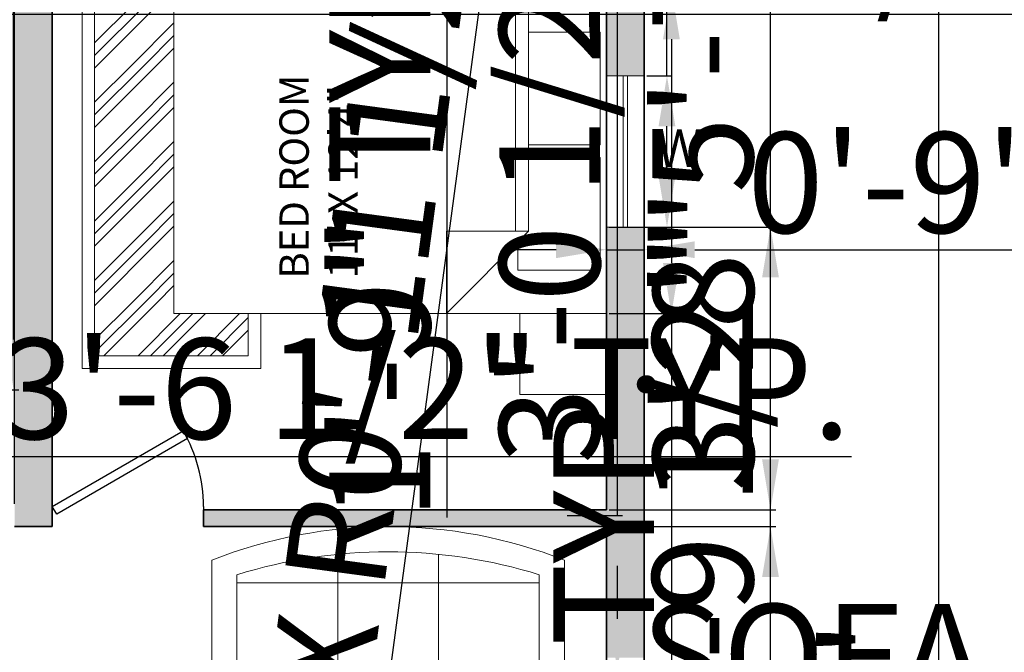
# Model space of a CAD drawing. Units: inches. Extents: x 830 to 1639, y 2591 to 3595.
# Tile 4 of 7: x 1133 to 1367, y 2957 to 3108. Entities that reach past the tile are written whole.
import ezdxf

# ---------------------------------------------------------------- set-up
doc = ezdxf.new("R2010")
doc.units = ezdxf.units.IN
doc.layers.get('0').update_dxf_attribs({"color": 250})
for name, color, linetype, lineweight in [('A-ANNO-DIMS', 2, 'Continuous', 18), ('A-ANNO-TEXT', 7, 'Continuous', 18), ('A-AREA-IDEN', 7, 'Continuous', 25), ('A-DOOR', 3, 'Continuous', 25), ('A-FLOR-PATT', 252, 'Continuous', 13), ('A-FURN', 8, 'Continuous', 18), ('A-GLAZ', 4, 'Continuous', 18), ('A-WALL', 7, 'Continuous', 35), ('A-WALL-PATT', 5, 'Continuous', 13), ('C-PROP', 7, 'Continuous', 35)]:
    doc.layers.add(name, color=color, linetype=linetype, lineweight=lineweight)
doc.styles.get("Standard").update_dxf_attribs({"font": 'arial.ttf'})
doc.dimstyles.new('ISO-25', dxfattribs={"dimtxt": 24, "dimasz": 12, "dimexe": 1.25, "dimexo": 0.625, "dimtad": 1, "dimdec": 0, "dimlunit": 3, "dimtxsty": 'Standard', "dimcen": 2.5, "dimadec": 0, "dimazin": 0, "dimtfac": 1, "dimtdec": 0, "dimtmove": 0, "dimatfit": 3, "dimfxl": 1, "dimarcsym": 0})

# ---------------------------------------------------------------- blocks, each defined once
blk = doc.blocks.new('Sofa - Roundback 7 ft.')
for p, q in [((-12.00002, -32.4421), (-12.00003, -6.5971)), ((11.99997, -32.4421), (11.99998, -6.5971)), ((-36.000027, -34), (-36.000027, -11.4696)), ((35.99998, -34), (35.99998, -11.4696)), ((-35.999844, -13.3819), (35.9998, -13.3819)), ((-36.000027, -32.4421), (35.99998, -32.4421))]:
    blk.add_line(p, q)
for points in [[(-36.000027, -34), (-42.000027, -34), (-42.000027, -8)], [(41.99998, -8), (41.99998, -34), (35.99998, -34)]]:
    blk.add_lwpolyline(points)
for centre, radius, start, end in [((0, -114.25), 114.25, 68.43141, 111.5686), ((-0.00001, -127.1968), 121.1968, 72.72033, 107.2797)]:
    blk.add_arc(centre, radius, start, end)
blk = doc.blocks.new('*U11')
for p, q in [((-750, 0), (-750, 100)), ((0, 0), (0, 100))]:
    blk.add_line(p, q)
blk.add_lwpolyline([(0, 0), (-649.5, -375), (-671.4, -337.1), (-21.9, 37.9)], close=True)
blk.add_arc((0, 0), 750, 180, 210)
blk = doc.blocks.new('Bed - Queen')
for p, q in [((0, -80.00003), (0, 0)), ((0, 0), (59.99999, 0)), ((59.99999, 0), (59.99999, -80.00003)), ((7.99999, -1.2), (28.79998, -1.2)), ((7.99999, -14.4), (7.99999, -1.2)), ((28.79998, -1.2), (28.79998, -14.4)), ((31.19999, -1.2), (51.99999, -1.2)), ((31.19999, -14.4), (31.19999, -1.2)), ((51.99999, -1.2), (51.99999, -16.4)), ((0, -14.4), (44.8, -14.4)), ((59.99999, -29.6), (44.8, -14.4)), ((44.8, -14.4), (44.8, -29.6)), ((44.8, -16.8), (0, -16.8)), ((51.99999, -16.4), (46.79936, -16.4)), ((44.8, -29.6), (59.99999, -29.6)), ((59.99999, -80.00003), (0, -80.00003))]:
    blk.add_line(p, q)
blk = doc.blocks.new('*D14')
at = {"layer": 'A-ANNO-DIMS', "color": 0, "lineweight": -2, "transparency": 16777216}
for p, q in [((1282.21, 3212.09), (1352.88, 3212.09)), ((1351.63, 3200.09), (1351.63, 2684.09)), ((1282.21, 2672.09), (1352.88, 2672.09))]:
    blk.add_line(p, q, dxfattribs=at)
at = {"layer": 'A-ANNO-DIMS', "color": 0, "transparency": 16777216}
for points in [[(1349.63, 3200.09), (1353.63, 3200.09), (1351.63, 3212.09)], [(1349.63, 2684.09), (1353.63, 2684.09), (1351.63, 2672.09)]]:
    blk.add_solid(points, dxfattribs=at)
at = {"layer": 'Defpoints', "color": 0, "transparency": 16777216}
for p in [(1281.59, 3212.09), (1281.59, 2672.09), (1351.63, 2672.09)]:
    blk.add_point(p, dxfattribs=at)
at = {"layer": 'A-ANNO-DIMS', "color": 0, "transparency": 16777216, "insert": (1338.8, 2942.09), "char_height": 24, "attachment_point": 5, "rotation": 90}
blk.add_mtext("45'", dxfattribs=at)
blk = doc.blocks.new('WIN-36IN')
for p, q in [((0, 0), (0, 36)), ((0, 36), (9, 36)), ((4, 0), (4, 36)), ((5, 36), (5, 0)), ((9, 36), (9, 0)), ((9, 0), (0, 0))]:
    blk.add_line(p, q)
blk = doc.blocks.new('BEDSIDE-TABLE')
blk.add_lwpolyline([(20.72, 0), (0, 0), (0, 19.25), (20.72, 19.25)], close=True)
blk = doc.blocks.new('BED-RUG-PLAN')
for points in [[(0, 92.63), (0, 105.69), (42.59, 105.69), (42.59, 0), (0, 0), (0, 15.31)], [(3, 92.63), (3, 102.69), (39.59, 102.69), (39.59, 3), (3, 3), (3, 15.31)]]:
    blk.add_lwpolyline(points)
blk = doc.blocks.new('*D22')
at = {"layer": 'A-ANNO-DIMS', "color": 0, "lineweight": -2, "transparency": 16777216}
for p, q in [((1286.99, 3094.42), (1286.99, 3411.37)), ((1282.21, 3094.42), (1288.24, 3094.42)), ((1286.99, 3070.42), (1286.99, 3082.42)), ((1282.21, 3058.42), (1288.24, 3058.42))]:
    blk.add_line(p, q, dxfattribs=at)
at = {"layer": 'A-ANNO-DIMS', "color": 0, "transparency": 16777216}
for points in [[(1284.99, 3082.42), (1288.99, 3082.42), (1286.99, 3094.42)], [(1284.99, 3070.42), (1288.99, 3070.42), (1286.99, 3058.42)]]:
    blk.add_solid(points, dxfattribs=at)
at = {"layer": 'Defpoints', "color": 0, "transparency": 16777216}
for p in [(1281.59, 3094.42), (1286.99, 3094.42), (1281.59, 3058.42)]:
    blk.add_point(p, dxfattribs=at)
at = {"layer": 'A-ANNO-DIMS', "color": 0, "transparency": 16777216, "insert": (1273.94, 3258.89), "char_height": 24, "attachment_point": 5, "rotation": 90}
blk.add_mtext('WINDOW 3\'-0" TYP.', dxfattribs=at)
blk = doc.blocks.new('*D23')
at = {"layer": 'A-ANNO-DIMS', "color": 0, "lineweight": -2, "transparency": 16777216}
for p, q in [((1272.59, 3057.79), (1272.59, 3051.77)), ((1281.59, 3057.79), (1281.59, 3051.77)), ((1260.59, 3053.02), (1248.59, 3053.02)), ((1272.59, 3053.02), (1281.59, 3053.02)), ((1293.59, 3053.02), (1453.13, 3053.02))]:
    blk.add_line(p, q, dxfattribs=at)
at = {"layer": 'A-ANNO-DIMS', "color": 0, "transparency": 16777216}
for points in [[(1260.59, 3055.02), (1260.59, 3051.02), (1272.59, 3053.02)], [(1293.59, 3055.02), (1293.59, 3051.02), (1281.59, 3053.02)]]:
    blk.add_solid(points, dxfattribs=at)
at = {"layer": 'Defpoints', "color": 0, "transparency": 16777216}
for p in [(1272.59, 3058.42), (1281.59, 3058.42), (1281.59, 3053.02)]:
    blk.add_point(p, dxfattribs=at)
at = {"layer": 'A-ANNO-DIMS', "color": 0, "transparency": 16777216, "insert": (1379.36, 3065.9), "char_height": 24, "attachment_point": 5}
blk.add_mtext('0\'-9" TYP.', dxfattribs=at)
blk = doc.blocks.new('*D26')
at = {"layer": 'A-ANNO-DIMS', "color": 0, "lineweight": -2, "transparency": 16777216}
for p, q in [((990.59, 3111.63), (990.59, 3107.9)), ((1011.31, 3111.63), (1011.31, 3107.9)), ((978.59, 3109.15), (966.59, 3109.15)), ((990.59, 3109.15), (1011.31, 3109.15)), ((1023.31, 3109.15), (1464.86, 3109.15))]:
    blk.add_line(p, q, dxfattribs=at)
at = {"layer": 'A-ANNO-DIMS', "color": 0, "transparency": 16777216}
for points in [[(978.59, 3111.15), (978.59, 3107.15), (990.59, 3109.15)], [(1023.31, 3111.15), (1023.31, 3107.15), (1011.31, 3109.15)]]:
    blk.add_solid(points, dxfattribs=at)
at = {"layer": 'Defpoints', "color": 0, "transparency": 16777216}
for p in [(990.59, 3112.26), (1011.31, 3112.26), (1011.31, 3109.15)]:
    blk.add_point(p, dxfattribs=at)
at = {"layer": 'A-ANNO-DIMS', "color": 0, "transparency": 16777216, "insert": (1250.08, 3122.18), "char_height": 24, "attachment_point": 5}
blk.add_mtext('NIGHTSTAND 1\'-8 1/2" TYP.', dxfattribs=at)
blk = doc.blocks.new('*D28')
at = {"layer": 'A-ANNO-DIMS', "color": 0, "lineweight": -2, "transparency": 16777216}
for p, q in [((1178.57, 2952.46), (1178.57, 2939.24)), ((1262.57, 2952.46), (1262.57, 2939.24)), ((1190.57, 2940.49), (1250.57, 2940.49)), ((1262.57, 2940.49), (1522.6, 2940.49))]:
    blk.add_line(p, q, dxfattribs=at)
at = {"layer": 'A-ANNO-DIMS', "color": 0, "transparency": 16777216}
for points in [[(1190.57, 2942.49), (1190.57, 2938.49), (1178.57, 2940.49)], [(1250.57, 2942.49), (1250.57, 2938.49), (1262.57, 2940.49)]]:
    blk.add_solid(points, dxfattribs=at)
at = {"layer": 'Defpoints', "color": 0, "transparency": 16777216}
for p in [(1178.57, 2953.09), (1262.57, 2953.09), (1262.57, 2940.49)]:
    blk.add_point(p, dxfattribs=at)
at = {"layer": 'A-ANNO-DIMS', "color": 0, "transparency": 16777216, "insert": (1398.58, 2953.53), "char_height": 24, "attachment_point": 5}
blk.add_mtext('SOFA 7\'-0" TYP.', dxfattribs=at)
blk = doc.blocks.new('*D29')
at = {"layer": 'A-ANNO-DIMS', "color": 0, "lineweight": -2, "transparency": 16777216}
for p, q in [((1275.17, 2989.75), (1275.17, 3205.2)), ((1263.19, 2989.75), (1276.42, 2989.75)), ((1275.17, 2965.09), (1275.17, 2977.75)), ((1263.19, 2953.09), (1276.42, 2953.09))]:
    blk.add_line(p, q, dxfattribs=at)
at = {"layer": 'A-ANNO-DIMS', "color": 0, "transparency": 16777216}
for points in [[(1273.17, 2977.75), (1277.17, 2977.75), (1275.17, 2989.75)], [(1273.17, 2965.09), (1277.17, 2965.09), (1275.17, 2953.09)]]:
    blk.add_solid(points, dxfattribs=at)
at = {"layer": 'Defpoints', "color": 0, "transparency": 16777216}
for p in [(1262.57, 2989.75), (1275.17, 2989.75), (1262.57, 2953.09)]:
    blk.add_point(p, dxfattribs=at)
at = {"layer": 'A-ANNO-DIMS', "color": 0, "transparency": 16777216, "insert": (1262.13, 3103.48), "char_height": 24, "attachment_point": 5, "rotation": 90}
blk.add_mtext('3\'-0 1/2" TYP.', dxfattribs=at)
blk = doc.blocks.new('*D31')
at = {"layer": 'A-ANNO-DIMS', "color": 0, "lineweight": -2, "transparency": 16777216}
for p, q in [((1234.59, 3191.58), (1234.59, 3203.58)), ((1238.92, 3179.58), (1233.34, 3179.58)), ((1234.59, 3179.58), (1234.59, 3158.58)), ((1238.92, 3158.58), (1233.34, 3158.58)), ((1234.59, 3146.58), (1234.59, 2989.29))]:
    blk.add_line(p, q, dxfattribs=at)
at = {"layer": 'A-ANNO-DIMS', "color": 0, "transparency": 16777216}
for points in [[(1232.59, 3191.58), (1236.59, 3191.58), (1234.59, 3179.58)], [(1232.59, 3146.58), (1236.59, 3146.58), (1234.59, 3158.58)]]:
    blk.add_solid(points, dxfattribs=at)
at = {"layer": 'Defpoints', "color": 0, "transparency": 16777216}
for p in [(1239.54, 3179.58), (1234.59, 3158.58), (1239.54, 3158.58)]:
    blk.add_point(p, dxfattribs=at)
at = {"layer": 'A-ANNO-DIMS', "color": 0, "transparency": 16777216, "insert": (1221.71, 3061.94), "char_height": 24, "attachment_point": 5, "rotation": 90}
blk.add_mtext('1\'-9" TYP.', dxfattribs=at)
blk = doc.blocks.new('*D36')
at = {"layer": 'A-ANNO-DIMS', "color": 0, "lineweight": -2, "transparency": 16777216}
for p, q in [((1169.49, 3115.77), (1169.49, 3131.86)), ((1272.59, 3115.77), (1272.59, 3131.86)), ((1181.49, 3130.61), (1260.59, 3130.61)), ((1272.59, 3130.61), (1638.88, 3130.61))]:
    blk.add_line(p, q, dxfattribs=at)
at = {"layer": 'A-ANNO-DIMS', "color": 0, "transparency": 16777216}
for points in [[(1181.49, 3132.61), (1181.49, 3128.61), (1169.49, 3130.61)], [(1260.59, 3132.61), (1260.59, 3128.61), (1272.59, 3130.61)]]:
    blk.add_solid(points, dxfattribs=at)
at = {"layer": 'Defpoints', "color": 0, "transparency": 16777216}
for p in [(1272.59, 3130.61), (1169.49, 3115.15), (1272.59, 3115.15)]:
    blk.add_point(p, dxfattribs=at)
at = {"layer": 'A-ANNO-DIMS', "color": 0, "transparency": 16777216, "insert": (1461.74, 3144.38), "char_height": 24, "attachment_point": 5}
blk.add_mtext('QUEEN BED 8\'-7" TYP.', dxfattribs=at)
blk = doc.blocks.new('*D37')
at = {"layer": 'A-ANNO-DIMS', "color": 0, "lineweight": -2, "transparency": 16777216}
for p, q in [((1273.21, 3115.15), (1289.3, 3115.15)), ((1288.05, 3103.15), (1288.05, 3049.83)), ((1273.21, 3037.83), (1289.3, 3037.83)), ((1288.05, 3037.83), (1288.05, 2822.23))]:
    blk.add_line(p, q, dxfattribs=at)
at = {"layer": 'A-ANNO-DIMS', "color": 0, "transparency": 16777216}
for points in [[(1286.05, 3103.15), (1290.05, 3103.15), (1288.05, 3115.15)], [(1286.05, 3049.83), (1290.05, 3049.83), (1288.05, 3037.83)]]:
    blk.add_solid(points, dxfattribs=at)
at = {"layer": 'Defpoints', "color": 0, "transparency": 16777216}
for p in [(1272.59, 3115.15), (1272.59, 3037.83), (1288.05, 3037.83)]:
    blk.add_point(p, dxfattribs=at)
at = {"layer": 'A-ANNO-DIMS', "color": 0, "transparency": 16777216, "insert": (1275.02, 2924.03), "char_height": 24, "attachment_point": 5, "rotation": 90}
blk.add_mtext('6\'-5 1/2" TYP.', dxfattribs=at)
blk = doc.blocks.new('*D39')
at = {"layer": 'A-ANNO-DIMS', "color": 0, "lineweight": -2, "transparency": 16777216}
for p, q in [((1209.62, 3142.46), (1209.62, 3139.14)), ((1220.27, 3142.46), (1220.27, 3139.14)), ((1197.62, 3140.39), (1185.62, 3140.39)), ((1209.62, 3140.39), (1220.27, 3140.39)), ((1232.27, 3140.39), (1466.38, 3140.39))]:
    blk.add_line(p, q, dxfattribs=at)
at = {"layer": 'A-ANNO-DIMS', "color": 0, "transparency": 16777216}
for points in [[(1197.62, 3142.39), (1197.62, 3138.39), (1209.62, 3140.39)], [(1232.27, 3142.39), (1232.27, 3138.39), (1220.27, 3140.39)]]:
    blk.add_solid(points, dxfattribs=at)
at = {"layer": 'Defpoints', "color": 0, "transparency": 16777216}
for p in [(1209.62, 3143.09), (1220.27, 3143.09), (1220.27, 3140.39)]:
    blk.add_point(p, dxfattribs=at)
at = {"layer": 'A-ANNO-DIMS', "color": 0, "transparency": 16777216, "insert": (1355.32, 3153.43), "char_height": 24, "attachment_point": 5}
blk.add_mtext('0\'-10 1/2" TYP.', dxfattribs=at)
blk = doc.blocks.new('*D40')
at = {"layer": 'A-ANNO-DIMS', "color": 0, "lineweight": -2, "transparency": 16777216}
for p, q in [((1131.38, 3125.32), (1131.38, 3423.36)), ((1116.15, 3125.32), (1132.63, 3125.32)), ((1131.38, 3031.63), (1131.38, 3113.32)), ((1116.15, 3019.63), (1132.63, 3019.63))]:
    blk.add_line(p, q, dxfattribs=at)
at = {"layer": 'A-ANNO-DIMS', "color": 0, "transparency": 16777216}
for points in [[(1129.38, 3113.32), (1133.38, 3113.32), (1131.38, 3125.32)], [(1129.38, 3031.63), (1133.38, 3031.63), (1131.38, 3019.63)]]:
    blk.add_solid(points, dxfattribs=at)
at = {"layer": 'Defpoints', "color": 0, "transparency": 16777216}
for p in [(1115.52, 3125.32), (1131.38, 3125.32), (1115.52, 3019.63)]:
    blk.add_point(p, dxfattribs=at)
at = {"layer": 'A-ANNO-DIMS', "color": 0, "transparency": 16777216, "insert": (1118.34, 3280.34), "char_height": 24, "attachment_point": 5, "rotation": 90}
blk.add_mtext('RUG 8\'-9 1/2" TYP.', dxfattribs=at)
blk = doc.blocks.new('*D41')
at = {"layer": 'A-ANNO-DIMS', "color": 0, "lineweight": -2, "transparency": 16777216}
for p, q in [((1072.93, 3019), (1072.93, 3002.53)), ((1115.52, 3019), (1115.52, 3002.53)), ((1084.93, 3003.78), (1103.52, 3003.78)), ((1115.52, 3003.78), (1330.97, 3003.78))]:
    blk.add_line(p, q, dxfattribs=at)
at = {"layer": 'A-ANNO-DIMS', "color": 0, "transparency": 16777216}
for points in [[(1084.93, 3005.78), (1084.93, 3001.78), (1072.93, 3003.78)], [(1103.52, 3005.78), (1103.52, 3001.78), (1115.52, 3003.78)]]:
    blk.add_solid(points, dxfattribs=at)
at = {"layer": 'Defpoints', "color": 0, "transparency": 16777216}
for p in [(1072.93, 3019.63), (1115.52, 3019.63), (1115.52, 3003.78)]:
    blk.add_point(p, dxfattribs=at)
at = {"layer": 'A-ANNO-DIMS', "color": 0, "transparency": 16777216, "insert": (1229.25, 3016.82), "char_height": 24, "attachment_point": 5}
blk.add_mtext('3\'-6 1/2" TYP.', dxfattribs=at)
blk = doc.blocks.new('*D49')
at = {"layer": 'A-ANNO-DIMS', "color": 0, "lineweight": -2, "transparency": 16777216}
for p, q in [((1095.59, 2991.71), (1095.59, 3243.39)), ((1131.59, 2992.51), (1131.59, 3243.39)), ((1107.59, 3242.14), (1119.59, 3242.14)), ((1131.59, 3242.14), (1208.62, 3242.14))]:
    blk.add_line(p, q, dxfattribs=at)
at = {"layer": 'A-ANNO-DIMS', "color": 0, "transparency": 16777216}
for points in [[(1107.59, 3244.14), (1107.59, 3240.14), (1095.59, 3242.14)], [(1119.59, 3244.14), (1119.59, 3240.14), (1131.59, 3242.14)]]:
    blk.add_solid(points, dxfattribs=at)
at = {"layer": 'Defpoints', "color": 0, "transparency": 16777216}
for p in [(1131.59, 3242.14), (1095.59, 2991.09), (1131.59, 2991.89)]:
    blk.add_point(p, dxfattribs=at)
at = {"layer": 'A-ANNO-DIMS', "color": 0, "transparency": 16777216, "insert": (1176.11, 3255.02), "char_height": 24, "attachment_point": 5}
blk.add_mtext('3\'-0"', dxfattribs=at)
blk = doc.blocks.new('*D57')
at = {"layer": 'A-ANNO-DIMS', "color": 0, "lineweight": -2, "transparency": 16777216}
for p, q in [((951.54, 2944.9), (951.54, 3077.67)), ((1203.59, 2944.9), (950.29, 2944.9)), ((951.54, 2864.53), (951.54, 2932.9)), ((1203.59, 2852.53), (950.29, 2852.53))]:
    blk.add_line(p, q, dxfattribs=at)
at = {"layer": 'A-ANNO-DIMS', "color": 0, "transparency": 16777216}
for points in [[(949.54, 2932.9), (953.54, 2932.9), (951.54, 2944.9)], [(949.54, 2864.53), (953.54, 2864.53), (951.54, 2852.53)]]:
    blk.add_solid(points, dxfattribs=at)
at = {"layer": 'Defpoints', "color": 0, "transparency": 16777216}
for p in [(951.54, 2944.9), (1204.22, 2944.9), (1204.22, 2852.53)]:
    blk.add_point(p, dxfattribs=at)
at = {"layer": 'A-ANNO-DIMS', "color": 0, "transparency": 16777216, "insert": (938.51, 3017.28), "char_height": 24, "attachment_point": 5, "rotation": 90}
blk.add_mtext('7\'-8 1/2"', dxfattribs=at)
blk = doc.blocks.new('*D63')
at = {"layer": 'A-ANNO-DIMS', "color": 0, "lineweight": -2, "transparency": 16777216}
for p, q in [((1311.64, 2919.85), (1311.64, 3053.23)), ((1282.21, 2919.85), (1312.89, 2919.85)), ((1311.64, 2898.33), (1311.64, 2907.85)), ((1282.21, 2886.33), (1312.89, 2886.33))]:
    blk.add_line(p, q, dxfattribs=at)
at = {"layer": 'A-ANNO-DIMS', "color": 0, "transparency": 16777216}
for points in [[(1309.64, 2907.85), (1313.64, 2907.85), (1311.64, 2919.85)], [(1309.64, 2898.33), (1313.64, 2898.33), (1311.64, 2886.33)]]:
    blk.add_solid(points, dxfattribs=at)
at = {"layer": 'Defpoints', "color": 0, "transparency": 16777216}
for p in [(1281.59, 2919.85), (1311.64, 2919.85), (1281.59, 2886.33)]:
    blk.add_point(p, dxfattribs=at)
at = {"layer": 'A-ANNO-DIMS', "color": 0, "transparency": 16777216, "insert": (1298.61, 2992.54), "char_height": 24, "attachment_point": 5, "rotation": 90}
blk.add_mtext('2\'-9 1/2"', dxfattribs=at)
blk = doc.blocks.new('*D67')
at = {"layer": 'A-ANNO-DIMS', "color": 0, "lineweight": -2, "transparency": 16777216}
for p, q in [((1311.64, 2987.09), (1311.64, 3064.12)), ((1273.21, 2987.09), (1312.89, 2987.09)), ((1311.64, 2955.04), (1311.64, 2975.09)), ((1265.21, 2943.04), (1312.89, 2943.04))]:
    blk.add_line(p, q, dxfattribs=at)
at = {"layer": 'A-ANNO-DIMS', "color": 0, "transparency": 16777216}
for points in [[(1309.64, 2975.09), (1313.64, 2975.09), (1311.64, 2987.09)], [(1309.64, 2955.04), (1313.64, 2955.04), (1311.64, 2943.04)]]:
    blk.add_solid(points, dxfattribs=at)
at = {"layer": 'Defpoints', "color": 0, "transparency": 16777216}
for p in [(1272.59, 2987.09), (1311.64, 2987.09), (1264.59, 2943.04)]:
    blk.add_point(p, dxfattribs=at)
at = {"layer": 'A-ANNO-DIMS', "color": 0, "transparency": 16777216, "insert": (1298.75, 3031.6), "char_height": 24, "attachment_point": 5, "rotation": 90}
blk.add_mtext('3\'-8"', dxfattribs=at)
blk = doc.blocks.new('*D68')
at = {"layer": 'A-ANNO-DIMS', "color": 0, "lineweight": -2, "transparency": 16777216}
for p, q in [((1311.64, 3058.42), (1311.64, 3191.39)), ((1273.21, 3058.42), (1312.89, 3058.42)), ((1311.64, 3003.09), (1311.64, 3046.42)), ((1273.21, 2991.09), (1312.89, 2991.09))]:
    blk.add_line(p, q, dxfattribs=at)
at = {"layer": 'A-ANNO-DIMS', "color": 0, "transparency": 16777216}
for points in [[(1309.64, 3046.42), (1313.64, 3046.42), (1311.64, 3058.42)], [(1309.64, 3003.09), (1313.64, 3003.09), (1311.64, 2991.09)]]:
    blk.add_solid(points, dxfattribs=at)
at = {"layer": 'Defpoints', "color": 0, "transparency": 16777216}
for p in [(1272.59, 3058.42), (1311.64, 3058.42), (1272.59, 2991.09)]:
    blk.add_point(p, dxfattribs=at)
at = {"layer": 'A-ANNO-DIMS', "color": 0, "transparency": 16777216, "insert": (1298.61, 3130.9), "char_height": 24, "attachment_point": 5, "rotation": 90}
blk.add_mtext('5\'-7 1/2"', dxfattribs=at)
blk = doc.blocks.new('*D76')
at = {"layer": 'A-ANNO-DIMS', "color": 0, "lineweight": -2, "transparency": 16777216}
for p, q in [((1250.77, 3173.28), (1249.26, 3162.05)), ((1217.52, 2925.89), (1247.66, 3150.16))]:
    blk.add_line(p, q, dxfattribs=at)
at = {"layer": 'A-ANNO-DIMS', "color": 0, "transparency": 16777216}
blk.add_solid([(1245.68, 3150.42), (1249.65, 3149.89), (1249.26, 3162.05)], dxfattribs=at)
at = {"layer": 'Defpoints', "color": 0, "transparency": 16777216}
for p in [(1250.77, 3173.28), (1249.26, 3162.05)]:
    blk.add_point(p, dxfattribs=at)
at = {"layer": 'A-ANNO-DIMS', "color": 0, "transparency": 16777216, "insert": (1218.87, 3033.81), "char_height": 24, "attachment_point": 5, "rotation": 82.3443}
blk.add_mtext('6X R0\'-11 1/2"', dxfattribs=at)

msp = doc.modelspace()

# ---------------------------------------------------------------- hatches: boundary and pattern name
at = {"layer": 'A-FLOR-PATT'}
h = msp.add_hatch(dxfattribs=at)
h.set_pattern_fill('GOST_GROUND', color=256)
h.paths.add_polyline_path([(1112.52, 3122.32), (1075.93, 3122.32), (1075.93, 3112.26), (1093.69, 3112.26), (1093.69, 3034.94), (1075.93, 3034.94), (1075.93, 3022.63), (1112.52, 3022.63)])
h.paths.add_polyline_path([(1169.49, 3115.15), (1187.25, 3115.15), (1187.25, 3127.45), (1150.65, 3127.45), (1150.65, 3027.77), (1187.25, 3027.77), (1187.25, 3037.83), (1169.49, 3037.83)])
h.paths.add_polyline_path([(1131.59, 3203.09), (1083.59, 3203.09), (1083.59, 3167.09), (1131.59, 3167.09)])
h.paths.add_polyline_path([(1188.59, 3203.09), (1140.59, 3203.09), (1140.59, 3167.09), (1188.59, 3167.09)])
at = {"layer": 'A-WALL-PATT'}
h = msp.add_hatch(color=256, dxfattribs=at)
h.dxf.hatch_style = 1
h.paths.add_polyline_path([(990.59, 3203.09), (1079.59, 3203.09), (1079.59, 3167.09), (1083.59, 3167.09), (1083.59, 3203.09), (1131.59, 3203.09), (1131.59, 2987.09), (1140.59, 2987.09), (1140.59, 2991.89), (1140.59, 3203.09), (1188.59, 3203.09), (1188.59, 3167.09), (1192.59, 3167.09), (1192.59, 3203.09), (1272.59, 3203.09), (1272.59, 3181.45), (1281.59, 3181.45), (1281.59, 3212.09), (981.59, 3212.09), (981.59, 3182.32), (990.59, 3182.32)])
h = msp.add_hatch(color=256, dxfattribs=at)
h.dxf.hatch_style = 1
h.paths.add_polyline_path([(1272.59, 3143.09), (1192.23, 3143.09), (1191.79, 3142.55), (1188.59, 3143.09), (1188.59, 3139.09), (1272.59, 3139.09), (1272.59, 3094.42), (1281.59, 3094.42), (1281.59, 3157.45), (1272.59, 3157.45)])
h = msp.add_hatch(color=256, dxfattribs=at)
h.dxf.hatch_style = 1
h.paths.add_polyline_path([(1281.59, 3058.42), (1272.59, 3058.42), (1272.59, 3037.83), (1272.63, 3037.83), (1272.63, 3018.58), (1272.59, 2991.09), (1176.59, 2991.09), (1176.59, 2987.09), (1272.59, 2987.09), (1272.59, 2955.85), (1281.59, 2955.85)])

# ---------------------------------------------------------------- linework, layer by layer
at = {"layer": 'A-WALL'}
for p, q in [((1140.59, 2991.09), (1140.59, 3203.09)), ((1140.59, 2987.09), (1140.59, 3139.09)), ((1272.59, 3139.09), (1272.59, 2991.09)), ((1272.59, 2991.09), (1272.59, 3139.09)), ((1176.59, 2987.09), (1176.59, 2991.09)), ((1272.59, 2987.09), (1272.59, 2810.09)), ((1272.59, 2810.09), (1272.59, 2987.09))]:
    msp.add_line(p, q, dxfattribs=at)
for points in [[(1176.59, 2991.09), (1272.59, 2991.09)], [(1131.59, 2987.09), (1140.59, 2987.09)], [(1176.59, 2987.09), (1272.59, 2987.09)]]:
    msp.add_lwpolyline(points, dxfattribs=at)
at = {"layer": 'C-PROP'}
msp.add_lwpolyline([(981.59, 3212.09), (1281.59, 3212.09), (1281.59, 2672.09), (981.59, 2672.09)], close=True, dxfattribs=at)

# ---------------------------------------------------------------- block references
at = {"layer": 'A-DOOR', "xscale": 0.0480000000000001, "yscale": 0.0480000000000001, "zscale": 0.0480000000000001, "rotation": 180}
msp.add_blockref('*U11', (1140.59, 2991.89), dxfattribs=at)
at = {"layer": 'A-FURN', "rotation": 180}
msp.add_blockref('BED-RUG-PLAN', (1190.25, 3130.45), dxfattribs=at)
at = {"layer": 'A-FURN', "xscale": 1.288695656948927, "yscale": 1.288695656948927, "zscale": 1.288695656948927, "rotation": 270}
msp.add_blockref('Bed - Queen', (1272.59, 3115.15), dxfattribs=at)
at = {"layer": 'A-FURN'}
for name, p in [('BEDSIDE-TABLE', (1251.92, 3018.58)), ('Sofa - Roundback 7 ft.', (1220.57, 2987.09))]:
    msp.add_blockref(name, p, dxfattribs=at)
at = {"layer": 'A-GLAZ'}
msp.add_blockref('WIN-36IN', (1272.59, 3058.42), dxfattribs=at)

# ---------------------------------------------------------------- texts
at = {"layer": 'A-ANNO-TEXT', "insert": (1284.52, 3081.69), "char_height": 9, "width": 31.3961, "attachment_point": 1}
msp.add_mtext('{\\fArial|b1|i0|c0|p34;W}', dxfattribs=at)
at = {"layer": 'A-AREA-IDEN', "insert": (1194.68, 3046.14), "char_height": 7, "width": 58.1932, "attachment_point": 1, "rotation": 90}
msp.add_mtext('{\\fArial|b1|i0|c0|p34;BED ROOM\\P11\' X 12\'4"}', dxfattribs=at)

# ---------------------------------------------------------------- dimensions: what is measured, and where the dimension line sits
at = {"layer": 'A-ANNO-DIMS'}
for base, p1, p2, angle, text, picture, middle in [((1131.38, 3125.32), (1115.52, 3019.63), (1115.52, 3125.32), 90, 'RUG <> TYP.', '*D40', (1118.34, 3280.34)), ((1286.99, 3094.42), (1281.59, 3058.42), (1281.59, 3094.42), 90, 'WINDOW <> TYP.', '*D22', (1273.94, 3258.89)), ((1234.59, 3158.58), (1239.54, 3179.58), (1239.54, 3158.58), 270, '<> TYP.', '*D31', (1221.71, 3061.94)), ((1275.17, 2989.75), (1262.57, 2953.09), (1262.57, 2989.75), 90, '<> TYP.', '*D29', (1262.13, 3103.48)), ((1288.05, 3037.83), (1272.59, 3115.15), (1272.59, 3037.83), 270, '<> TYP.', '*D37', (1275.02, 2924.03))]:
    dim = msp.add_linear_dim(base=base, p1=p1, p2=p2, angle=angle, text=text, dimstyle='ISO-25', override={"dimdec": 1, "dimlfac": 1, "dimrnd": 0, "dimzin": 1, "dimdsep": 46, "dimlunit": 4, "dimfrac": 2}, dxfattribs=at)
    dim.commit()
    dim.dimension.update_dxf_attribs({"geometry": picture, "text_midpoint": middle})
dim = msp.add_linear_dim(base=(1131.59, 3242.14), p1=(1095.59, 2991.09), p2=(1131.59, 2991.89), dimstyle='ISO-25', override={"dimdec": 1, "dimlfac": 1, "dimrnd": 0, "dimzin": 1, "dimdsep": 46, "dimlunit": 4, "dimfrac": 2}, dxfattribs=at)
dim.commit()
dim.dimension.update_dxf_attribs({"geometry": '*D49', "text_midpoint": (1176.11, 3255.02)})
for base, p1, p2, text, picture, middle in [((1272.59, 3130.61), (1169.49, 3115.15), (1272.59, 3115.15), 'QUEEN BED <> TYP.', '*D36', (1461.74, 3144.38)), ((1220.2661, 3140.394), (1209.616, 3143.0874), (1220.2661, 3143.0874), '<> TYP.', '*D39', (1355.3222, 3153.4283)), ((1011.31, 3109.15), (990.59, 3112.26), (1011.31, 3112.26), 'NIGHTSTAND <> TYP.', '*D26', (1250.08, 3122.18)), ((1281.59, 3053.02), (1272.59, 3058.42), (1281.59, 3058.42), '<> TYP.', '*D23', (1379.36, 3065.9)), ((1115.52, 3003.78), (1072.93, 3019.63), (1115.52, 3019.63), '<> TYP.', '*D41', (1229.25, 3016.82)), ((1262.57, 2940.49), (1178.57, 2953.09), (1262.57, 2953.09), 'SOFA <> TYP.', '*D28', (1398.58, 2953.53))]:
    dim = msp.add_linear_dim(base=base, p1=p1, p2=p2, text=text, dimstyle='ISO-25', override={"dimdec": 1, "dimlfac": 1, "dimrnd": 0, "dimzin": 1, "dimdsep": 46, "dimlunit": 4, "dimfrac": 2}, dxfattribs=at)
    dim.commit()
    dim.dimension.update_dxf_attribs({"geometry": picture, "text_midpoint": middle})
for base, p1, p2, override, picture, middle in [((1351.63, 2672.09), (1281.59, 3212.09), (1281.59, 2672.09), {"dimclrd": 0, "dimclre": 0, "dimclrt": 0}, '*D14', (1338.8, 2942.09)), ((1311.64, 3058.42), (1272.59, 2991.09), (1272.59, 3058.42), {"dimdec": 1, "dimlfac": 1, "dimrnd": 0, "dimzin": 1, "dimdsep": 46, "dimlunit": 4, "dimfrac": 2}, '*D68', (1298.61, 3130.9)), ((951.54, 2944.9), (1204.22, 2852.53), (1204.22, 2944.9), {"dimdec": 1, "dimlfac": 1, "dimrnd": 0, "dimzin": 1, "dimdsep": 46, "dimlunit": 4, "dimfrac": 2}, '*D57', (938.51, 3017.28)), ((1311.6397, 2987.0874), (1264.5897, 2943.038), (1272.5897, 2987.0874), {"dimdec": 1, "dimlfac": 1, "dimrnd": 0, "dimzin": 1, "dimdsep": 46, "dimlunit": 4, "dimfrac": 2}, '*D67', (1298.7528, 3031.6033)), ((1311.64, 2919.85), (1281.59, 2886.33), (1281.59, 2919.85), {"dimdec": 1, "dimlfac": 1, "dimrnd": 0, "dimzin": 1, "dimdsep": 46, "dimlunit": 4, "dimfrac": 2}, '*D63', (1298.61, 2992.54))]:
    dim = msp.add_linear_dim(base=base, p1=p1, p2=p2, angle=90, dimstyle='ISO-25', override=override, dxfattribs=at)
    dim.commit()
    dim.dimension.update_dxf_attribs({"geometry": picture, "text_midpoint": middle})
dim = msp.add_radius_dim(center=(1250.77, 3173.28), mpoint=(1249.26, 3162.05), text='6X <>', dimstyle='ISO-25', override={"dimdec": 1, "dimlfac": 1, "dimrnd": 0, "dimzin": 1, "dimdsep": 46, "dimlunit": 4, "dimfrac": 2}, dxfattribs=at)
dim.commit()
dim.dimension.update_dxf_attribs({"geometry": '*D76', "text_midpoint": (1218.87, 3033.81)})

doc.saveas('drawing.dxf')
